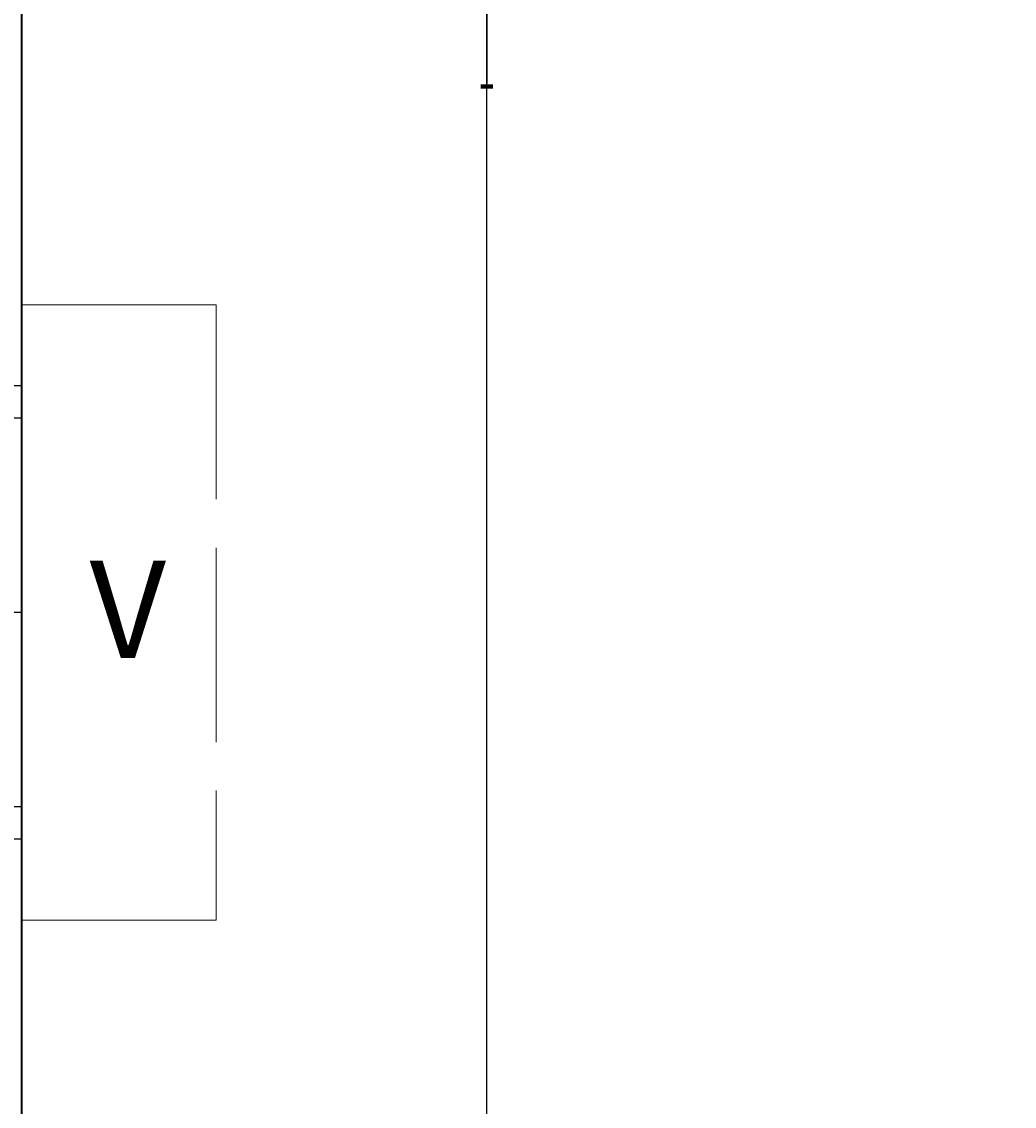
# Model space of a CAD drawing. Units: inches. Extents: x -301 to 715, y -607 to 364.
# Tile 99 of 141: x 133 to 194, y -77 to -10. Entities that reach past the tile are written whole.
import ezdxf

# ---------------------------------------------------------------- set-up
doc = ezdxf.new("R2010")
doc.units = ezdxf.units.IN
doc.header["$MEASUREMENT"] = 0
doc.linetypes.add('ACAD_ISO02W100', pattern=[15, 12, -3])
for name, color, linetype, lineweight in [('A-ANNO-DIMS', 2, 'Continuous', 18), ('A-ANNO-TEXT', 4, 'Continuous', 18), ('A-GLAZ', 2, 'Continuous', 25), ('A-GLAZ-OVHD', 2, 'ACAD_ISO02W100', 18), ('A-WALL', 3, 'Continuous', 40)]:
    doc.layers.add(name, color=color, linetype=linetype, lineweight=lineweight)
doc.styles.get("Standard").update_dxf_attribs({"font": 'arial.ttf'})
doc.dimstyles.get("Standard").update_dxf_attribs({"dimtxt": 0.18, "dimasz": 0.18, "dimexe": 0.18, "dimexo": 0.0625, "dimgap": 0.09, "dimtad": 0, "dimtih": 1, "dimtoh": 1, "dimdec": 1, "dimzin": 0, "dimdsep": 46, "dimlunit": 4, "dimtxsty": 'Standard', "dimcen": 0.09, "dimclrd": 3, "dimclre": 4, "dimclrt": 6, "dimadec": 0, "dimazin": 0, "dimtfac": 1, "dimtdec": 1, "dimtofl": 0, "dimtmove": 0, "dimatfit": 3, "dimfxl": 1, "dimtfill": 2, "dimtfillclr": 51, "dimtolj": 1, "dimtzin": 0, "dimarcsym": 0})

# ---------------------------------------------------------------- blocks, each defined once
blk = doc.blocks.new('VENT-24-PLAN')
for p, q in [((0, 0), (0, 9)), ((2, 0), (2, 9)), ((14, 0), (14, 9)), ((26, 0), (26, 9)), ((28, 0), (28, 9)), ((26, 5.5), (2, 5.5)), ((26, 3.5), (2, 3.5))]:
    blk.add_line(p, q)
blk = doc.blocks.new('VENT-SHADE-38')
for p, q in [((0, 0), (0, 12)), ((0, 12), (38, 12)), ((38, 0), (38, 12)), ((5, 0), (0, 0)), ((33, 0), (38, 0))]:
    blk.add_line(p, q)
blk = doc.blocks.new('*D162')
at = {"layer": 'A-ANNO-DIMS', "color": 4, "lineweight": -2, "transparency": 16777216}
for p, q in [((222.328, 320.182), (161.439, 320.182)), ((222.328, -233.818), (161.439, -233.818))]:
    blk.add_line(p, q, dxfattribs=at)
at = {"layer": 'A-ANNO-DIMS', "color": 3, "lineweight": -2, "transparency": 16777216}
for p, q in [((161.619, 320.002), (161.619, 43.364)), ((161.619, -233.638), (161.619, 43))]:
    blk.add_line(p, q, dxfattribs=at)
at = {"layer": 'A-ANNO-DIMS', "color": 3, "transparency": 16777216}
for points in [[(161.589, 320.002), (161.649, 320.002), (161.619, 320.182)], [(161.589, -233.638), (161.649, -233.638), (161.619, -233.818)]]:
    blk.add_solid(points, dxfattribs=at)
at = {"layer": 'Defpoints', "color": 0, "transparency": 16777216}
for p in [(161.619, 320.182), (222.39, 320.182), (222.39, -233.818)]:
    blk.add_point(p, dxfattribs=at)
at = {"layer": 'A-ANNO-DIMS', "color": 6, "transparency": 16777216, "insert": (161.619, 43.182), "char_height": 0.18, "attachment_point": 5, "bg_fill": 1, "box_fill_scale": 1.25, "bg_fill_color": 51, "bg_fill_transparency": 0}
blk.add_mtext('\\A1;46\'-2"', dxfattribs=at)
blk = doc.blocks.new('*D168')
at = {"layer": 'A-ANNO-DIMS', "color": 4, "lineweight": -2, "transparency": 16777216}
for p, q in [((222.328, 55.682), (161.439, 55.682)), ((222.328, -83.318), (161.439, -83.318))]:
    blk.add_line(p, q, dxfattribs=at)
at = {"layer": 'A-ANNO-DIMS', "color": 3, "lineweight": -2, "transparency": 16777216}
for p, q in [((161.619, 55.502), (161.619, -13.637)), ((161.619, -83.138), (161.619, -13.998))]:
    blk.add_line(p, q, dxfattribs=at)
at = {"layer": 'A-ANNO-DIMS', "color": 3, "transparency": 16777216}
for points in [[(161.589, 55.502), (161.649, 55.502), (161.619, 55.682)], [(161.589, -83.138), (161.649, -83.138), (161.619, -83.318)]]:
    blk.add_solid(points, dxfattribs=at)
at = {"layer": 'Defpoints', "color": 0, "transparency": 16777216}
for p in [(161.619, 55.682), (222.39, 55.682), (222.39, -83.318)]:
    blk.add_point(p, dxfattribs=at)
at = {"layer": 'A-ANNO-DIMS', "color": 6, "transparency": 16777216, "insert": (161.619, -13.818), "char_height": 0.18, "attachment_point": 5, "bg_fill": 1, "box_fill_scale": 1.25, "bg_fill_color": 51, "bg_fill_transparency": 0}
blk.add_mtext('\\A1;11\'-7"', dxfattribs=at)

msp = doc.modelspace()

# ---------------------------------------------------------------- linework, layer by layer
at = {"layer": 'A-WALL'}
for p, q in [((132.897, -9.818), (132.897, 199.182)), ((132.897, -76.818), (132.897, -9.818)), ((132.897, -124.818), (132.897, -76.818))]:
    msp.add_line(p, q, dxfattribs=at)

# ---------------------------------------------------------------- block references
at = {"layer": 'A-GLAZ', "rotation": 89.99999999999955}
msp.add_blockref('VENT-24-PLAN', (132.897, -60.318), dxfattribs=at)
at = {"layer": 'A-GLAZ-OVHD', "rotation": 269.9999999999998}
msp.add_blockref('VENT-SHADE-38', (132.896, -27.318), dxfattribs=at)

# ---------------------------------------------------------------- texts
at = {"layer": 'A-ANNO-TEXT'}
msp.add_text('V', height=6, dxfattribs=at).set_placement((137.092, -49.121))

# ---------------------------------------------------------------- dimensions: what is measured, and where the dimension line sits
at = {"layer": 'A-ANNO-DIMS'}
for base, p1, p2, picture, middle in [((161.619, 320.182), (222.39, -233.818), (222.39, 320.182), '*D162', (161.619, 43.182)), ((161.619, 55.682), (222.39, -83.318), (222.39, 55.682), '*D168', (161.619, -13.818))]:
    dim = msp.add_linear_dim(base=base, p1=p1, p2=p2, angle=90, dimstyle='Standard', override={"dimdec": 1, "dimlfac": 1, "dimrnd": 0, "dimzin": 1, "dimdsep": 46, "dimlunit": 4, "dimfrac": 2}, dxfattribs=at)
    dim.commit()
    dim.dimension.update_dxf_attribs({"geometry": picture, "text_midpoint": middle})

doc.saveas('drawing.dxf')
